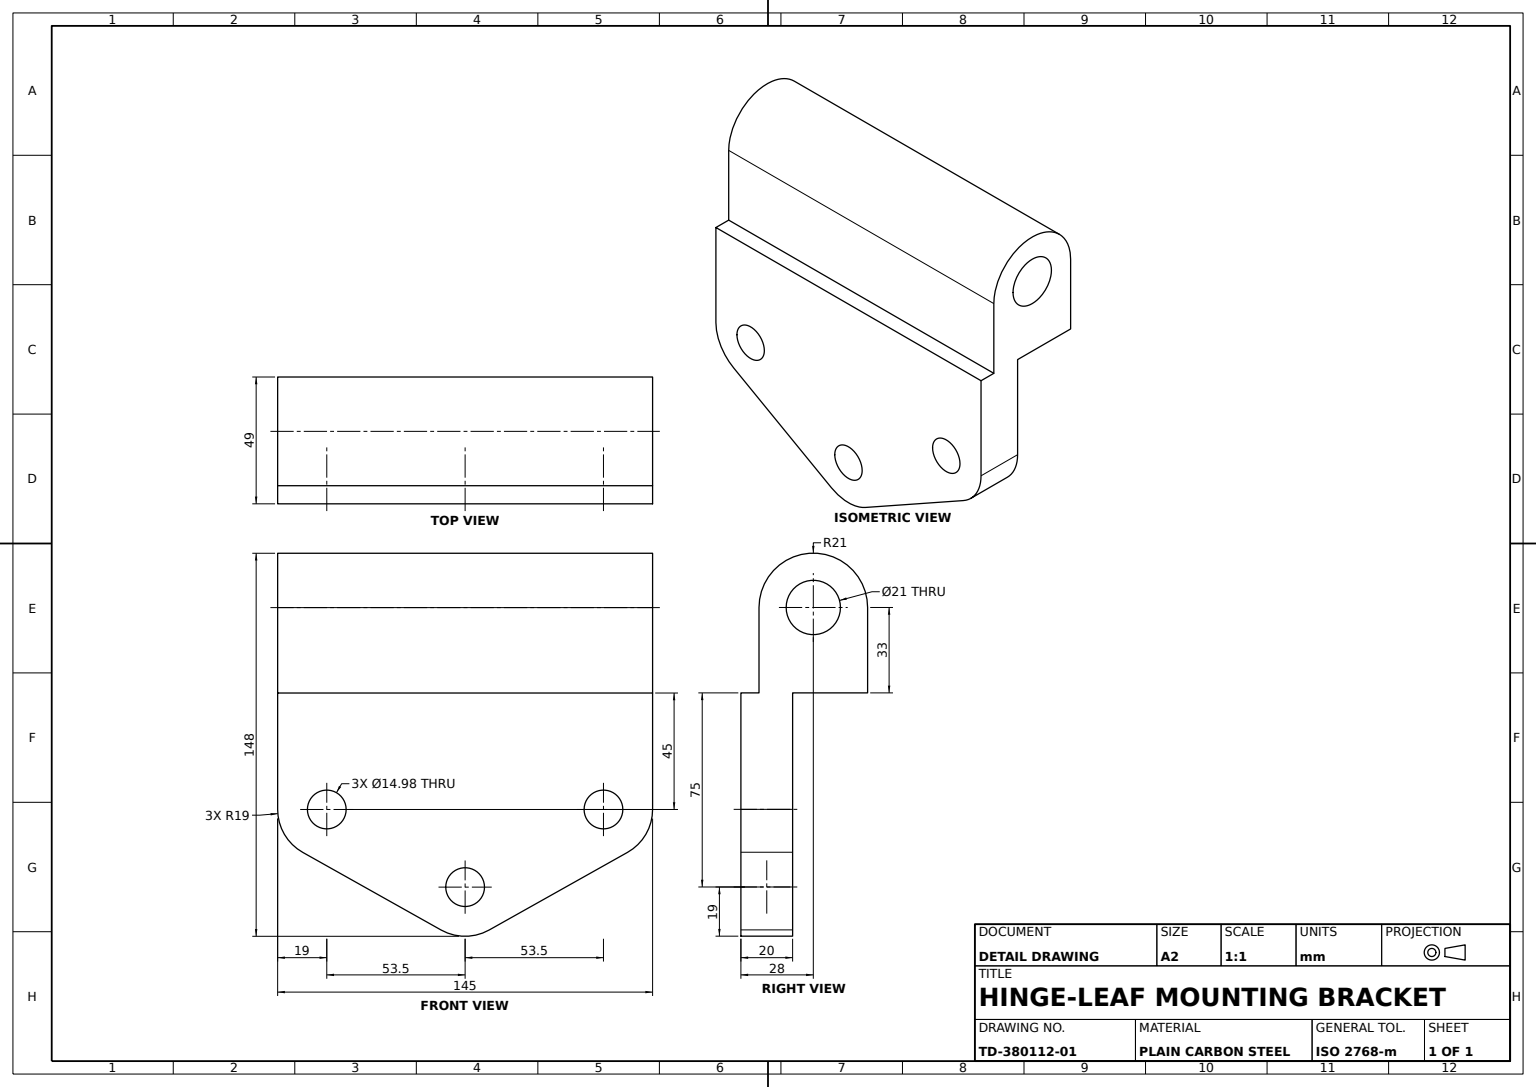
from build123d import *

# Parameters (mm, degrees)
BASE_PLATE_PROFILE_R      = 7.492267371
BASE_PLATE_20MM_DEPTH     = 20
HINGE_KNUCKLE_PROFILE_R   = 10.5
HINGE_KNUCKLE_145MM_DEPTH = 72.5


with BuildPart() as part:
    # Base Plate Profile → Base Plate 20mm (new body)
    with BuildSketch(Plane.XY):
        with BuildLine():
            Line((-72.5, 28.064546487), (72.5, 28.064546487))
            Line((72.5, 28.064546487), (72.5, -16.935453513))
            ThreePointArc((72.5, -16.935453513), (69.894587599, -26.538447706), (62.792895003, -33.507782934))
            Line((62.792895003, -33.507782934), (9.292895003, -63.507782934))
            ThreePointArc((9.292895003, -63.507782934), (0, -65.935453513), (-9.292895003, -63.507782934))
            Line((-9.292895003, -63.507782934), (-62.792895003, -33.507782934))
            ThreePointArc((-62.792895003, -33.507782934), (-69.894587599, -26.538447706), (-72.5, -16.935453513))
            Line((-72.5, -16.935453513), (-72.5, 28.064546487))
        make_face()
        with Locations((0, -46.935453513)):
            Circle(BASE_PLATE_PROFILE_R, mode=Mode.SUBTRACT)
        with Locations((53.5, -16.935453513)):
            Circle(BASE_PLATE_PROFILE_R, mode=Mode.SUBTRACT)
        with Locations((-53.5, -16.935453513)):
            Circle(BASE_PLATE_PROFILE_R, mode=Mode.SUBTRACT)
    extrude(amount=BASE_PLATE_20MM_DEPTH)

    # Hinge Knuckle Profile → Hinge Knuckle 145mm (add, symmetric)
    with BuildSketch(Plane(origin=(0, 0, 0), x_dir=(0, 0, -1), z_dir=(1, 0, 0))):
        with BuildLine():
            Line((29, 61.064546487), (29, 28.064546487))
            Line((29, 28.064546487), (-13, 28.064546487))
            Line((-13, 28.064546487), (-13, 61.064546487))
            ThreePointArc((-13, 61.064546487), (8, 82.064546487), (29, 61.064546487))
        make_face()
        with Locations((8, 61.064546487)):
            Circle(HINGE_KNUCKLE_PROFILE_R, mode=Mode.SUBTRACT)
    extrude(amount=HINGE_KNUCKLE_145MM_DEPTH, both=True)


solid = part.part
